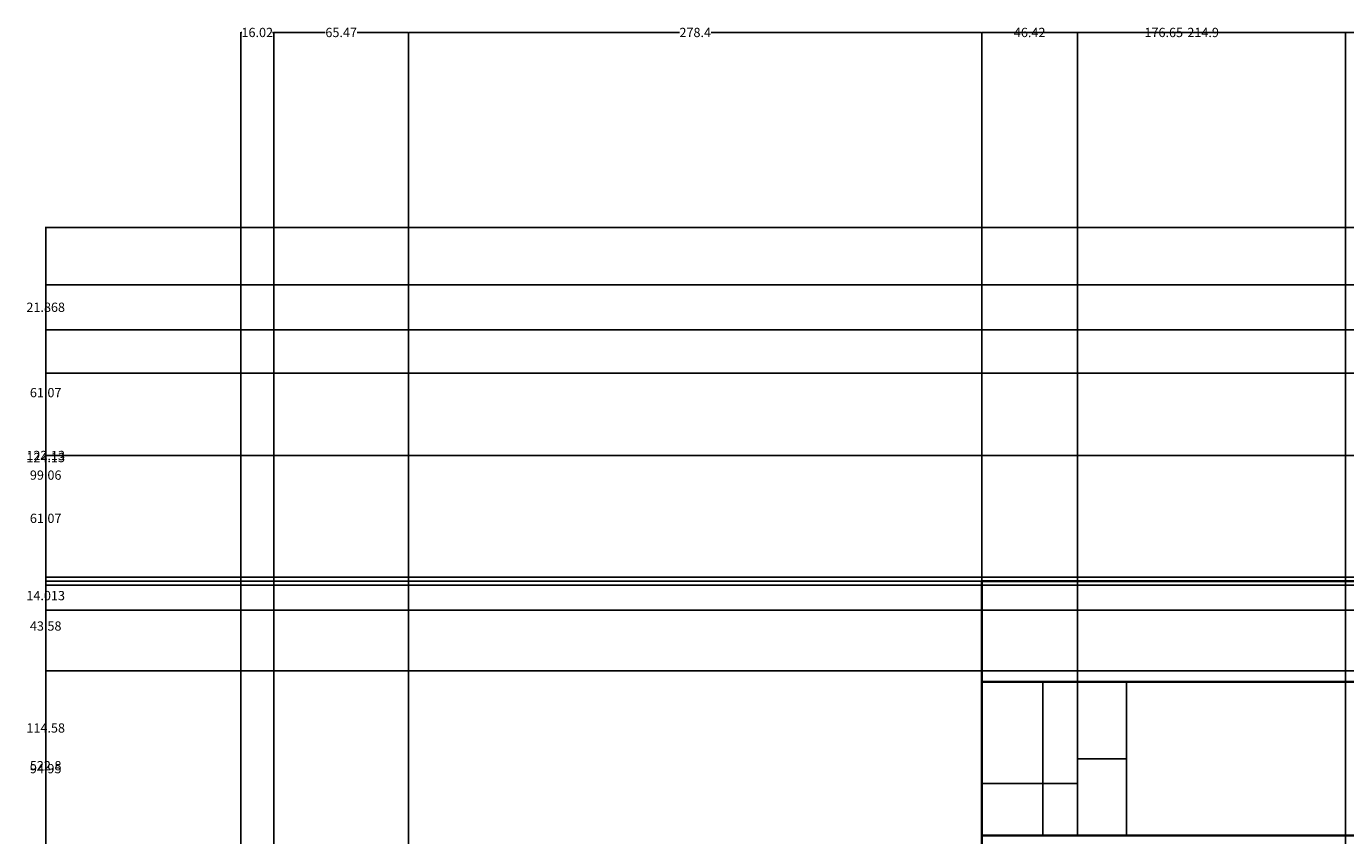
# Model space of a CAD drawing. Units: inches. Extents: x -1308 to 780, y 304 to 1023.
# Tile 2 of 7: x -1308 to -667, y 629 to 1023. Entities that reach past the tile are written whole.
import ezdxf

# ---------------------------------------------------------------- set-up
doc = ezdxf.new("R2010")
doc.units = ezdxf.units.IN
doc.header["$MEASUREMENT"] = 0
for name, color, linetype, lineweight in [('A-ANNO-DIMS', 2, 'Continuous', 18), ('A-ELEV', 7, 'Continuous', 35), ('A-GLAZ', 4, 'Continuous', 25)]:
    doc.layers.add(name, color=color, linetype=linetype, lineweight=lineweight)
doc.styles.get("Standard").update_dxf_attribs({"font": 'arial.ttf'})
doc.dimstyles.get("Standard").update_dxf_attribs({"dimtxt": 4.5, "dimasz": 0.18, "dimexe": 0.18, "dimexo": 0.0625, "dimgap": 0.09, "dimtad": 0, "dimtih": 1, "dimtoh": 1, "dimdec": 4, "dimzin": 0, "dimdsep": 46, "dimlunit": 4, "dimtxsty": 'Standard', "dimcen": 0.09, "dimadec": 0, "dimazin": 0, "dimtfac": 1, "dimtdec": 4, "dimtofl": 0, "dimtmove": 0, "dimatfit": 3, "dimfxl": 1, "dimtolj": 1, "dimtzin": 0, "dimarcsym": 0})

# ---------------------------------------------------------------- blocks, each defined once
blk = doc.blocks.new('*D2')
at = {"layer": 'A-ANNO-DIMS', "color": 0, "lineweight": -2, "transparency": 16777216}
for p, q in [((-1203.52, 521.91), (-1203.52, 1019.77)), ((-1203.34, 1019.59), (-1202.96, 1019.59)), ((-1187.68, 1019.59), (-1188.06, 1019.59)), ((-1187.5, 521.91), (-1187.5, 1019.77))]:
    blk.add_line(p, q, dxfattribs=at)
at = {"layer": 'A-ANNO-DIMS', "color": 0, "transparency": 16777216}
for points in [[(-1203.34, 1019.62), (-1203.34, 1019.56), (-1203.52, 1019.59)], [(-1187.68, 1019.62), (-1187.68, 1019.56), (-1187.5, 1019.59)]]:
    blk.add_solid(points, dxfattribs=at)
at = {"layer": 'Defpoints', "color": 0, "transparency": 16777216}
for p in [(-1187.5, 1019.59), (-1203.52, 521.84), (-1187.5, 521.84)]:
    blk.add_point(p, dxfattribs=at)
at = {"layer": 'A-ANNO-DIMS', "color": 0, "transparency": 16777216, "insert": (-1195.51, 1019.59), "char_height": 4.5, "attachment_point": 5}
blk.add_mtext('\\A1;16.02', dxfattribs=at)
blk = doc.blocks.new('*D3')
at = {"layer": 'A-ANNO-DIMS', "color": 0, "lineweight": -2, "transparency": 16777216}
for p, q in [((-1187.5, 521.91), (-1187.5, 1019.77)), ((-1187.32, 1019.59), (-1162.46, 1019.59)), ((-1122.2, 1019.59), (-1147.07, 1019.59)), ((-1122.02, 557.57), (-1122.02, 1019.77))]:
    blk.add_line(p, q, dxfattribs=at)
at = {"layer": 'A-ANNO-DIMS', "color": 0, "transparency": 16777216}
for points in [[(-1187.32, 1019.62), (-1187.32, 1019.56), (-1187.5, 1019.59)], [(-1122.2, 1019.62), (-1122.2, 1019.56), (-1122.02, 1019.59)]]:
    blk.add_solid(points, dxfattribs=at)
at = {"layer": 'Defpoints', "color": 0, "transparency": 16777216}
for p in [(-1122.02, 1019.59), (-1122.02, 557.51), (-1187.5, 521.84)]:
    blk.add_point(p, dxfattribs=at)
at = {"layer": 'A-ANNO-DIMS', "color": 0, "transparency": 16777216, "insert": (-1154.76, 1019.59), "char_height": 4.5, "attachment_point": 5}
blk.add_mtext('\\A1;65.47', dxfattribs=at)
blk = doc.blocks.new('*D4')
at = {"layer": 'A-ANNO-DIMS', "color": 0, "lineweight": -2, "transparency": 16777216}
for p, q in [((-1122.02, 557.57), (-1122.02, 1019.77)), ((-1121.84, 1019.59), (-990.52, 1019.59)), ((-843.78, 1019.59), (-975.1, 1019.59)), ((-843.6, 557.57), (-843.6, 1019.77))]:
    blk.add_line(p, q, dxfattribs=at)
at = {"layer": 'A-ANNO-DIMS', "color": 0, "transparency": 16777216}
for points in [[(-1121.84, 1019.62), (-1121.84, 1019.56), (-1122.02, 1019.59)], [(-843.78, 1019.62), (-843.78, 1019.56), (-843.6, 1019.59)]]:
    blk.add_solid(points, dxfattribs=at)
at = {"layer": 'Defpoints', "color": 0, "transparency": 16777216}
for p in [(-843.6, 1019.59), (-1122.02, 557.51), (-843.6, 557.51)]:
    blk.add_point(p, dxfattribs=at)
at = {"layer": 'A-ANNO-DIMS', "color": 0, "transparency": 16777216, "insert": (-982.81, 1019.59), "char_height": 4.5, "attachment_point": 5}
blk.add_mtext('\\A1;278.4', dxfattribs=at)
blk = doc.blocks.new('*D5')
at = {"layer": 'A-ANNO-DIMS', "color": 0, "lineweight": -2, "transparency": 16777216}
for p, q in [((-843.6, 402.08), (-843.6, 1019.77)), ((-843.42, 1019.59), (-764.51, 1019.59)), ((-667.13, 1019.59), (-746.04, 1019.59)), ((-666.95, 585.1), (-666.95, 1019.77))]:
    blk.add_line(p, q, dxfattribs=at)
at = {"layer": 'A-ANNO-DIMS', "color": 0, "transparency": 16777216}
for points in [[(-843.42, 1019.62), (-843.42, 1019.56), (-843.6, 1019.59)], [(-667.13, 1019.62), (-667.13, 1019.56), (-666.95, 1019.59)]]:
    blk.add_solid(points, dxfattribs=at)
at = {"layer": 'Defpoints', "color": 0, "transparency": 16777216}
for p in [(-666.95, 1019.59), (-666.95, 585.04), (-843.6, 402.02)]:
    blk.add_point(p, dxfattribs=at)
at = {"layer": 'A-ANNO-DIMS', "color": 0, "transparency": 16777216, "insert": (-755.27, 1019.59), "char_height": 4.5, "attachment_point": 5}
blk.add_mtext('\\A1;176.65', dxfattribs=at)
blk = doc.blocks.new('*D6')
at = {"layer": 'A-ANNO-DIMS', "color": 0, "lineweight": -2, "transparency": 16777216}
for p, q in [((-666.95, 585.1), (-666.95, 1019.77)), ((-666.77, 1019.59), (-519.19, 1019.59)), ((-356.24, 1019.59), (-503.82, 1019.59)), ((-356.06, 585.1), (-356.06, 1019.77))]:
    blk.add_line(p, q, dxfattribs=at)
at = {"layer": 'A-ANNO-DIMS', "color": 0, "transparency": 16777216}
for points in [[(-666.77, 1019.62), (-666.77, 1019.56), (-666.95, 1019.59)], [(-356.24, 1019.62), (-356.24, 1019.56), (-356.06, 1019.59)]]:
    blk.add_solid(points, dxfattribs=at)
at = {"layer": 'Defpoints', "color": 0, "transparency": 16777216}
for p in [(-356.06, 1019.59), (-666.95, 585.04), (-356.06, 585.04)]:
    blk.add_point(p, dxfattribs=at)
at = {"layer": 'A-ANNO-DIMS', "color": 0, "transparency": 16777216, "insert": (-511.5, 1019.59), "char_height": 4.5, "attachment_point": 5}
blk.add_mtext('\\A1;310.9', dxfattribs=at)
blk = doc.blocks.new('*D17')
at = {"layer": 'A-ANNO-DIMS', "color": 0, "lineweight": -2, "transparency": 16777216}
for p, q in [((-843.6, 753.1), (-843.6, 1019.77)), ((-843.42, 1019.59), (-743.87, 1019.59)), ((-628.86, 1019.59), (-728.41, 1019.59)), ((-628.68, 753.1), (-628.68, 1019.77))]:
    blk.add_line(p, q, dxfattribs=at)
at = {"layer": 'A-ANNO-DIMS', "color": 0, "transparency": 16777216}
for points in [[(-843.42, 1019.62), (-843.42, 1019.56), (-843.6, 1019.59)], [(-628.86, 1019.62), (-628.86, 1019.56), (-628.68, 1019.59)]]:
    blk.add_solid(points, dxfattribs=at)
at = {"layer": 'Defpoints', "color": 0, "transparency": 16777216}
for p in [(-628.68, 1019.59), (-843.6, 753.04), (-628.68, 753.04)]:
    blk.add_point(p, dxfattribs=at)
at = {"layer": 'A-ANNO-DIMS', "color": 0, "transparency": 16777216, "insert": (-736.14, 1019.59), "char_height": 4.5, "attachment_point": 5}
blk.add_mtext('\\A1;214.9', dxfattribs=at)
blk = doc.blocks.new('*D48')
at = {"layer": 'A-ANNO-DIMS', "color": 0, "lineweight": -2, "transparency": 16777216}
for p, q in [((-843.6, 704.15), (-843.6, 1019.77)), ((-843.42, 1019.59), (-609.19, 1019.59)), ((-359.42, 1019.59), (-593.66, 1019.59)), ((-359.24, 704.15), (-359.24, 1019.77))]:
    blk.add_line(p, q, dxfattribs=at)
at = {"layer": 'A-ANNO-DIMS', "color": 0, "transparency": 16777216}
for points in [[(-843.42, 1019.62), (-843.42, 1019.56), (-843.6, 1019.59)], [(-359.42, 1019.62), (-359.42, 1019.56), (-359.24, 1019.59)]]:
    blk.add_solid(points, dxfattribs=at)
at = {"layer": 'Defpoints', "color": 0, "transparency": 16777216}
for p in [(-359.24, 1019.59), (-843.6, 704.09), (-359.24, 704.09)]:
    blk.add_point(p, dxfattribs=at)
at = {"layer": 'A-ANNO-DIMS', "color": 0, "transparency": 16777216, "insert": (-601.42, 1019.59), "char_height": 4.5, "attachment_point": 5}
blk.add_mtext('\\A1;484.4', dxfattribs=at)
blk = doc.blocks.new('*D50')
at = {"layer": 'A-ANNO-DIMS', "color": 0, "lineweight": -2, "transparency": 16777216}
for p, q in [((-843.6, 654.76), (-843.6, 1019.77)), ((-843.42, 1019.59), (-828.14, 1019.59)), ((-797.36, 1019.59), (-812.64, 1019.59)), ((-797.18, 654.76), (-797.18, 1019.77))]:
    blk.add_line(p, q, dxfattribs=at)
at = {"layer": 'A-ANNO-DIMS', "color": 0, "transparency": 16777216}
for points in [[(-843.42, 1019.62), (-843.42, 1019.56), (-843.6, 1019.59)], [(-797.36, 1019.62), (-797.36, 1019.56), (-797.18, 1019.59)]]:
    blk.add_solid(points, dxfattribs=at)
at = {"layer": 'Defpoints', "color": 0, "transparency": 16777216}
for p in [(-797.18, 1019.59), (-843.6, 654.7), (-797.18, 654.7)]:
    blk.add_point(p, dxfattribs=at)
at = {"layer": 'A-ANNO-DIMS', "color": 0, "transparency": 16777216, "insert": (-820.39, 1019.59), "char_height": 4.5, "attachment_point": 5}
blk.add_mtext('\\A1;46.42', dxfattribs=at)
blk = doc.blocks.new('*D57')
at = {"layer": 'A-ANNO-DIMS', "color": 0, "lineweight": -2, "transparency": 16777216}
for p, q in [((-628.74, 924.84), (-1298.45, 924.84)), ((-1298.27, 924.66), (-1298.27, 665.82)), ((-1298.27, 402.2), (-1298.27, 661.04)), ((-1203.58, 402.02), (-1298.45, 402.02))]:
    blk.add_line(p, q, dxfattribs=at)
at = {"layer": 'A-ANNO-DIMS', "color": 0, "transparency": 16777216}
for points in [[(-1298.3, 924.66), (-1298.24, 924.66), (-1298.27, 924.84)], [(-1298.3, 402.2), (-1298.24, 402.2), (-1298.27, 402.02)]]:
    blk.add_solid(points, dxfattribs=at)
at = {"layer": 'Defpoints', "color": 0, "transparency": 16777216}
for p in [(-1298.27, 924.84), (-628.68, 924.84), (-1203.52, 402.02)]:
    blk.add_point(p, dxfattribs=at)
at = {"layer": 'A-ANNO-DIMS', "color": 0, "transparency": 16777216, "insert": (-1298.27, 663.43), "char_height": 4.5, "attachment_point": 5}
blk.add_mtext('\\A1;522.8', dxfattribs=at)
blk = doc.blocks.new('*D64')
at = {"layer": 'A-ANNO-DIMS', "color": 0, "lineweight": -2, "transparency": 16777216}
for p, q in [((-843.54, 704.09), (771.09, 704.09)), ((770.91, 703.91), (770.91, 669.15)), ((770.91, 629.62), (770.91, 664.38)), ((-843.54, 629.44), (771.09, 629.44))]:
    blk.add_line(p, q, dxfattribs=at)
at = {"layer": 'A-ANNO-DIMS', "color": 0, "transparency": 16777216}
for points in [[(770.88, 703.91), (770.94, 703.91), (770.91, 704.09)], [(770.88, 629.62), (770.94, 629.62), (770.91, 629.44)]]:
    blk.add_solid(points, dxfattribs=at)
at = {"layer": 'Defpoints', "color": 0, "transparency": 16777216}
for p in [(-843.6, 704.09), (770.91, 704.09), (-843.6, 629.44)]:
    blk.add_point(p, dxfattribs=at)
at = {"layer": 'A-ANNO-DIMS', "color": 0, "transparency": 16777216, "insert": (770.91, 666.76), "char_height": 4.5, "attachment_point": 5}
blk.add_mtext('\\A1;74.64', dxfattribs=at)
blk = doc.blocks.new('*D65')
at = {"layer": 'A-ANNO-DIMS', "color": 0, "lineweight": -2, "transparency": 16777216}
for p, q in [((-843.54, 753.04), (771.09, 753.04)), ((770.91, 752.86), (770.91, 730.95)), ((770.91, 704.27), (770.91, 726.17)), ((-843.54, 704.09), (771.09, 704.09))]:
    blk.add_line(p, q, dxfattribs=at)
at = {"layer": 'A-ANNO-DIMS', "color": 0, "transparency": 16777216}
for points in [[(770.88, 752.86), (770.94, 752.86), (770.91, 753.04)], [(770.88, 704.27), (770.94, 704.27), (770.91, 704.09)]]:
    blk.add_solid(points, dxfattribs=at)
at = {"layer": 'Defpoints', "color": 0, "transparency": 16777216}
for p in [(-843.6, 753.04), (770.91, 753.04), (-843.6, 704.09)]:
    blk.add_point(p, dxfattribs=at)
at = {"layer": 'A-ANNO-DIMS', "color": 0, "transparency": 16777216, "insert": (770.91, 728.56), "char_height": 4.5, "attachment_point": 5}
blk.add_mtext('\\A1;48.95', dxfattribs=at)
blk = doc.blocks.new('*D69')
at = {"layer": 'A-ANNO-DIMS', "color": 0, "lineweight": -2, "transparency": 16777216}
for p, q in [((-271.41, 739.03), (-1298.45, 739.03)), ((-1298.27, 738.85), (-1298.27, 684.12)), ((-1298.27, 624.62), (-1298.27, 679.35)), ((-271.41, 624.44), (-1298.45, 624.44))]:
    blk.add_line(p, q, dxfattribs=at)
at = {"layer": 'A-ANNO-DIMS', "color": 0, "transparency": 16777216}
for points in [[(-1298.3, 738.85), (-1298.24, 738.85), (-1298.27, 739.03)], [(-1298.3, 624.62), (-1298.24, 624.62), (-1298.27, 624.44)]]:
    blk.add_solid(points, dxfattribs=at)
at = {"layer": 'Defpoints', "color": 0, "transparency": 16777216}
for p in [(-1298.27, 739.03), (-271.35, 739.03), (-271.35, 624.44)]:
    blk.add_point(p, dxfattribs=at)
at = {"layer": 'A-ANNO-DIMS', "color": 0, "transparency": 16777216, "insert": (-1298.27, 681.73), "char_height": 4.5, "attachment_point": 5}
blk.add_mtext('\\A1;114.58', dxfattribs=at)
blk = doc.blocks.new('*D70')
at = {"layer": 'A-ANNO-DIMS', "color": 0, "lineweight": -2, "transparency": 16777216}
for p, q in [((-271.41, 753.04), (-1298.45, 753.04)), ((-1298.27, 752.86), (-1298.27, 748.42)), ((-1298.27, 739.21), (-1298.27, 743.64)), ((-271.41, 739.03), (-1298.45, 739.03))]:
    blk.add_line(p, q, dxfattribs=at)
at = {"layer": 'A-ANNO-DIMS', "color": 0, "transparency": 16777216}
for points in [[(-1298.3, 752.86), (-1298.24, 752.86), (-1298.27, 753.04)], [(-1298.3, 739.21), (-1298.24, 739.21), (-1298.27, 739.03)]]:
    blk.add_solid(points, dxfattribs=at)
at = {"layer": 'Defpoints', "color": 0, "transparency": 16777216}
for p in [(-1298.27, 753.04), (-271.35, 753.04), (-271.35, 739.03)]:
    blk.add_point(p, dxfattribs=at)
at = {"layer": 'A-ANNO-DIMS', "color": 0, "transparency": 16777216, "insert": (-1298.27, 746.03), "char_height": 4.5, "attachment_point": 5}
blk.add_mtext('\\A1;14.013', dxfattribs=at)
blk = doc.blocks.new('*D71')
at = {"layer": 'A-ANNO-DIMS', "color": 0, "lineweight": -2, "transparency": 16777216}
for p, q in [((-271.41, 875.17), (-1298.45, 875.17)), ((-1298.27, 874.99), (-1298.27, 816.49)), ((-1298.27, 753.22), (-1298.27, 811.72)), ((-271.41, 753.04), (-1298.45, 753.04))]:
    blk.add_line(p, q, dxfattribs=at)
at = {"layer": 'A-ANNO-DIMS', "color": 0, "transparency": 16777216}
for points in [[(-1298.3, 874.99), (-1298.24, 874.99), (-1298.27, 875.17)], [(-1298.3, 753.22), (-1298.24, 753.22), (-1298.27, 753.04)]]:
    blk.add_solid(points, dxfattribs=at)
at = {"layer": 'Defpoints', "color": 0, "transparency": 16777216}
for p in [(-1298.27, 875.17), (-271.35, 875.17), (-271.35, 753.04)]:
    blk.add_point(p, dxfattribs=at)
at = {"layer": 'A-ANNO-DIMS', "color": 0, "transparency": 16777216, "insert": (-1298.27, 814.1), "char_height": 4.5, "attachment_point": 5}
blk.add_mtext('\\A1;122.13', dxfattribs=at)
blk = doc.blocks.new('*D72')
at = {"layer": 'A-ANNO-DIMS', "color": 0, "lineweight": -2, "transparency": 16777216}
for p, q in [((-271.41, 897.04), (-1298.45, 897.04)), ((-1298.27, 896.86), (-1298.27, 888.49)), ((-1298.27, 875.35), (-1298.27, 883.72)), ((-271.41, 875.17), (-1298.45, 875.17))]:
    blk.add_line(p, q, dxfattribs=at)
at = {"layer": 'A-ANNO-DIMS', "color": 0, "transparency": 16777216}
for points in [[(-1298.3, 896.86), (-1298.24, 896.86), (-1298.27, 897.04)], [(-1298.3, 875.35), (-1298.24, 875.35), (-1298.27, 875.17)]]:
    blk.add_solid(points, dxfattribs=at)
at = {"layer": 'Defpoints', "color": 0, "transparency": 16777216}
for p in [(-1298.27, 897.04), (-271.35, 897.04), (-271.35, 875.17)]:
    blk.add_point(p, dxfattribs=at)
at = {"layer": 'A-ANNO-DIMS', "color": 0, "transparency": 16777216, "insert": (-1298.27, 886.1), "char_height": 4.5, "attachment_point": 5}
blk.add_mtext('\\A1;21.868', dxfattribs=at)
blk = doc.blocks.new('*D82')
at = {"layer": 'A-ANNO-DIMS', "color": 0, "lineweight": -2, "transparency": 16777216}
for p, q in [((-25.92, 709.46), (-1298.45, 709.46)), ((-1298.27, 709.28), (-1298.27, 664.37)), ((-1298.27, 614.69), (-1298.27, 659.6)), ((-25.92, 614.51), (-1298.45, 614.51))]:
    blk.add_line(p, q, dxfattribs=at)
at = {"layer": 'A-ANNO-DIMS', "color": 0, "transparency": 16777216}
for points in [[(-1298.3, 709.28), (-1298.24, 709.28), (-1298.27, 709.46)], [(-1298.3, 614.69), (-1298.24, 614.69), (-1298.27, 614.51)]]:
    blk.add_solid(points, dxfattribs=at)
at = {"layer": 'Defpoints', "color": 0, "transparency": 16777216}
for p in [(-1298.27, 709.46), (-25.86, 709.46), (-25.86, 614.51)]:
    blk.add_point(p, dxfattribs=at)
at = {"layer": 'A-ANNO-DIMS', "color": 0, "transparency": 16777216, "insert": (-1298.27, 661.98), "char_height": 4.5, "attachment_point": 5}
blk.add_mtext('\\A1;94.95', dxfattribs=at)
blk = doc.blocks.new('*D83')
at = {"layer": 'A-ANNO-DIMS', "color": 0, "lineweight": -2, "transparency": 16777216}
for p, q in [((4.02, 753.04), (-1298.45, 753.04)), ((-1298.27, 752.86), (-1298.27, 733.64)), ((-1298.27, 709.64), (-1298.27, 728.86)), ((-25.92, 709.46), (-1298.45, 709.46))]:
    blk.add_line(p, q, dxfattribs=at)
at = {"layer": 'A-ANNO-DIMS', "color": 0, "transparency": 16777216}
for points in [[(-1298.3, 752.86), (-1298.24, 752.86), (-1298.27, 753.04)], [(-1298.3, 709.64), (-1298.24, 709.64), (-1298.27, 709.46)]]:
    blk.add_solid(points, dxfattribs=at)
at = {"layer": 'Defpoints', "color": 0, "transparency": 16777216}
for p in [(-1298.27, 753.04), (4.08, 753.04), (-25.86, 709.46)]:
    blk.add_point(p, dxfattribs=at)
at = {"layer": 'A-ANNO-DIMS', "color": 0, "transparency": 16777216, "insert": (-1298.27, 731.25), "char_height": 4.5, "attachment_point": 5}
blk.add_mtext('\\A1;43.58', dxfattribs=at)
blk = doc.blocks.new('*D84')
at = {"layer": 'A-ANNO-DIMS', "color": 0, "lineweight": -2, "transparency": 16777216}
for p, q in [((-292.51, 854.09), (-1298.45, 854.09)), ((-1298.27, 853.91), (-1298.27, 806.95)), ((-1298.27, 755.22), (-1298.27, 802.18)), ((-292.51, 755.04), (-1298.45, 755.04))]:
    blk.add_line(p, q, dxfattribs=at)
at = {"layer": 'A-ANNO-DIMS', "color": 0, "transparency": 16777216}
for points in [[(-1298.3, 853.91), (-1298.24, 853.91), (-1298.27, 854.09)], [(-1298.3, 755.22), (-1298.24, 755.22), (-1298.27, 755.04)]]:
    blk.add_solid(points, dxfattribs=at)
at = {"layer": 'Defpoints', "color": 0, "transparency": 16777216}
for p in [(-1298.27, 854.09), (-292.45, 854.09), (-292.45, 755.04)]:
    blk.add_point(p, dxfattribs=at)
at = {"layer": 'A-ANNO-DIMS', "color": 0, "transparency": 16777216, "insert": (-1298.27, 804.57), "char_height": 4.5, "attachment_point": 5}
blk.add_mtext('\\A1;99.06', dxfattribs=at)
blk = doc.blocks.new('*D85')
at = {"layer": 'A-ANNO-DIMS', "color": 0, "lineweight": -2, "transparency": 16777216}
for p, q in [((-63.07, 875.17), (-1298.45, 875.17)), ((-1298.27, 874.99), (-1298.27, 815.49)), ((-1298.27, 751.22), (-1298.27, 810.72)), ((-65.07, 751.04), (-1298.45, 751.04))]:
    blk.add_line(p, q, dxfattribs=at)
at = {"layer": 'A-ANNO-DIMS', "color": 0, "transparency": 16777216}
for points in [[(-1298.3, 874.99), (-1298.24, 874.99), (-1298.27, 875.17)], [(-1298.3, 751.22), (-1298.24, 751.22), (-1298.27, 751.04)]]:
    blk.add_solid(points, dxfattribs=at)
at = {"layer": 'Defpoints', "color": 0, "transparency": 16777216}
for p in [(-1298.27, 875.17), (-63.01, 875.17), (-65.01, 751.04)]:
    blk.add_point(p, dxfattribs=at)
at = {"layer": 'A-ANNO-DIMS', "color": 0, "transparency": 16777216, "insert": (-1298.27, 813.1), "char_height": 4.5, "attachment_point": 5}
blk.add_mtext('\\A1;124.13', dxfattribs=at)
blk = doc.blocks.new('*D86')
at = {"layer": 'A-ANNO-DIMS', "color": 0, "lineweight": -2, "transparency": 16777216}
for p, q in [((79.34, 814.1), (-1298.45, 814.1)), ((-1298.27, 813.92), (-1298.27, 785.96)), ((-1298.27, 753.22), (-1298.27, 781.18)), ((79.34, 753.04), (-1298.45, 753.04))]:
    blk.add_line(p, q, dxfattribs=at)
at = {"layer": 'A-ANNO-DIMS', "color": 0, "transparency": 16777216}
for points in [[(-1298.3, 813.92), (-1298.24, 813.92), (-1298.27, 814.1)], [(-1298.3, 753.22), (-1298.24, 753.22), (-1298.27, 753.04)]]:
    blk.add_solid(points, dxfattribs=at)
at = {"layer": 'Defpoints', "color": 0, "transparency": 16777216}
for p in [(-1298.27, 814.1), (79.41, 814.1), (79.41, 753.04)]:
    blk.add_point(p, dxfattribs=at)
at = {"layer": 'A-ANNO-DIMS', "color": 0, "transparency": 16777216, "insert": (-1298.27, 783.57), "char_height": 4.5, "attachment_point": 5}
blk.add_mtext('\\A1;61.07', dxfattribs=at)
blk = doc.blocks.new('*D87')
at = {"layer": 'A-ANNO-DIMS', "color": 0, "lineweight": -2, "transparency": 16777216}
for p, q in [((110.86, 875.17), (-1298.45, 875.17)), ((-1298.27, 874.99), (-1298.27, 847.03)), ((-1298.27, 814.28), (-1298.27, 842.25)), ((79.34, 814.1), (-1298.45, 814.1))]:
    blk.add_line(p, q, dxfattribs=at)
at = {"layer": 'A-ANNO-DIMS', "color": 0, "transparency": 16777216}
for points in [[(-1298.3, 874.99), (-1298.24, 874.99), (-1298.27, 875.17)], [(-1298.3, 814.28), (-1298.24, 814.28), (-1298.27, 814.1)]]:
    blk.add_solid(points, dxfattribs=at)
at = {"layer": 'Defpoints', "color": 0, "transparency": 16777216}
for p in [(-1298.27, 875.17), (110.92, 875.17), (79.41, 814.1)]:
    blk.add_point(p, dxfattribs=at)
at = {"layer": 'A-ANNO-DIMS', "color": 0, "transparency": 16777216, "insert": (-1298.27, 844.64), "char_height": 4.5, "attachment_point": 5}
blk.add_mtext('\\A1;61.07', dxfattribs=at)

msp = doc.modelspace()

# ---------------------------------------------------------------- linework, layer by layer
at = {"layer": 'A-ELEV'}
for p, q in [((-843.5988, 704.0857), (-843.5988, 753.0385)), ((-843.5988, 753.0385), (-628.6809, 753.0385)), ((-359.2437, 704.0857), (-843.5988, 704.0857)), ((-843.5988, 704.0857), (-843.5988, 629.4421)), ((-843.5988, 402.0158), (-843.5988, 629.4421)), ((-843.5988, 629.4421), (-390.5363, 629.4421))]:
    msp.add_line(p, q, dxfattribs=at)
at = {"layer": 'A-GLAZ'}
for p, q in [((-813.9606, 704.0857), (-813.9606, 629.4421)), ((-797.1797, 704.0857), (-797.1797, 629.4421)), ((-773.441, 704.0857), (-773.441, 629.4421)), ((-797.1797, 666.7639), (-773.441, 666.7639)), ((-843.5988, 654.7004), (-797.1797, 654.7004))]:
    msp.add_line(p, q, dxfattribs=at)

# ---------------------------------------------------------------- dimensions: what is measured, and where the dimension line sits
at = {"layer": 'A-ANNO-DIMS'}
for base, p1, p2, override, picture, middle in [((-1187.498, 1019.5921), (-1203.518, 521.8442), (-1187.498, 521.8442), {"dimdec": 2, "dimlfac": 1, "dimrnd": 0, "dimzin": 0, "dimdsep": 46, "dimlunit": 2}, '*D2', (-1195.508, 1019.5921)), ((-1122.0239, 1019.5921), (-1187.498, 521.8442), (-1122.0239, 557.5099), {"dimdec": 2, "dimlfac": 1, "dimrnd": 0, "dimzin": 0, "dimdsep": 46, "dimlunit": 2}, '*D3', (-1154.761, 1019.5921)), ((-843.5988, 1019.5921), (-1122.0239, 557.5099), (-843.5988, 557.5099), {"dimdec": 1, "dimlfac": 1, "dimrnd": 0, "dimzin": 0, "dimdsep": 46, "dimlunit": 2}, '*D4', (-982.8114, 1019.5921)), ((-666.946, 1019.5921), (-843.5988, 402.0158), (-666.946, 585.0385), {"dimdec": 2, "dimlfac": 1, "dimrnd": 0, "dimzin": 0, "dimdsep": 46, "dimlunit": 2}, '*D5', (-755.2724, 1019.5921)), ((-628.6809, 1019.5921), (-843.5988, 753.0385), (-628.6809, 753.0385), {"dimdec": 1, "dimlfac": 1, "dimrnd": 0, "dimzin": 0, "dimdsep": 46, "dimlunit": 2}, '*D17', (-736.1398, 1019.5921)), ((-359.2437, 1019.5921), (-843.5988, 704.0857), (-359.2437, 704.0857), {"dimdec": 1, "dimlfac": 1, "dimrnd": 0, "dimzin": 0, "dimdsep": 46, "dimlunit": 2}, '*D48', (-601.4212, 1019.5921)), ((-797.1797, 1019.5921), (-843.5988, 654.7004), (-797.1797, 654.7004), {"dimdec": 2, "dimlfac": 1, "dimrnd": 0, "dimzin": 0, "dimdsep": 46, "dimlunit": 2}, '*D50', (-820.3892, 1019.5921)), ((-356.0562, 1019.5921), (-666.946, 585.0385), (-356.0562, 585.0385), {"dimdec": 1, "dimlfac": 1, "dimrnd": 0, "dimzin": 0, "dimdsep": 46, "dimlunit": 2}, '*D6', (-511.5011, 1019.5921))]:
    dim = msp.add_linear_dim(base=base, p1=p1, p2=p2, dimstyle='Standard', override=override, dxfattribs=at)
    dim.commit()
    dim.dimension.update_dxf_attribs({"geometry": picture, "text_midpoint": middle})
for base, p1, p2, override, picture, middle in [((-1298.268, 924.8421), (-1203.518, 402.0158), (-628.6809, 924.8421), {"dimdec": 1, "dimlfac": 1, "dimrnd": 0, "dimzin": 0, "dimdsep": 46, "dimlunit": 2}, '*D57', (-1298.268, 663.429)), ((-1298.268, 897.0385), (-271.346, 875.1709), (-271.346, 897.0385), {"dimdec": 3, "dimlfac": 1, "dimrnd": 0, "dimzin": 0, "dimdsep": 46, "dimlunit": 2}, '*D72', (-1298.268, 886.1047)), ((-1298.268, 875.1709), (-271.346, 753.0385), (-271.346, 875.1709), {"dimdec": 2, "dimlfac": 1, "dimrnd": 0, "dimzin": 0, "dimdsep": 46, "dimlunit": 2}, '*D71', (-1298.268, 814.1047)), ((-1298.268, 875.1709), (-65.0069, 751.0385), (-63.0069, 875.1709), {"dimdec": 2, "dimlfac": 1, "dimrnd": 0, "dimzin": 0, "dimdsep": 46, "dimlunit": 2}, '*D85', (-1298.268, 813.1047)), ((-1298.268, 875.1709), (79.4055, 814.1047), (110.9181, 875.1709), {"dimdec": 2, "dimlfac": 1, "dimrnd": 0, "dimzin": 0, "dimdsep": 46, "dimlunit": 2}, '*D87', (-1298.268, 844.6378)), ((-1298.268, 854.0948), (-292.4461, 755.0385), (-292.4461, 854.0948), {"dimdec": 2, "dimlfac": 1, "dimrnd": 0, "dimzin": 0, "dimdsep": 46, "dimlunit": 2}, '*D84', (-1298.268, 804.5667)), ((-1298.268, 814.1047), (79.4055, 753.0385), (79.4055, 814.1047), {"dimdec": 2, "dimlfac": 1, "dimrnd": 0, "dimzin": 0, "dimdsep": 46, "dimlunit": 2}, '*D86', (-1298.268, 783.5716)), ((-1298.268, 753.0385), (-271.346, 739.0259), (-271.346, 753.0385), {"dimdec": 3, "dimlfac": 1, "dimrnd": 0, "dimzin": 0, "dimdsep": 46, "dimlunit": 2}, '*D70', (-1298.268, 746.0322)), ((-1298.268, 753.0385), (-25.8575, 709.4602), (4.0783, 753.0385), {"dimdec": 2, "dimlfac": 1, "dimrnd": 0, "dimzin": 0, "dimdsep": 46, "dimlunit": 2}, '*D83', (-1298.268, 731.2494)), ((770.9076, 753.0385), (-843.5988, 704.0857), (-843.5988, 753.0385), {"dimdec": 2, "dimlfac": 1, "dimrnd": 0, "dimzin": 0, "dimdsep": 46, "dimlunit": 2}, '*D65', (770.9076, 728.5621)), ((-1298.268, 739.0259), (-271.346, 624.4429), (-271.346, 739.0259), {"dimdec": 2, "dimlfac": 1, "dimrnd": 0, "dimzin": 0, "dimdsep": 46, "dimlunit": 2}, '*D69', (-1298.268, 681.7344)), ((-1298.268, 709.4602), (-25.8575, 614.5069), (-25.8575, 709.4602), {"dimdec": 2, "dimlfac": 1, "dimrnd": 0, "dimzin": 0, "dimdsep": 46, "dimlunit": 2}, '*D82', (-1298.268, 661.9835)), ((770.9076, 704.0857), (-843.5988, 629.4421), (-843.5988, 704.0857), {"dimdec": 2, "dimlfac": 1, "dimrnd": 0, "dimzin": 0, "dimdsep": 46, "dimlunit": 2}, '*D64', (770.9076, 666.7639))]:
    dim = msp.add_linear_dim(base=base, p1=p1, p2=p2, angle=90, dimstyle='Standard', override=override, dxfattribs=at)
    dim.commit()
    dim.dimension.update_dxf_attribs({"geometry": picture, "text_midpoint": middle})

doc.saveas('drawing.dxf')
